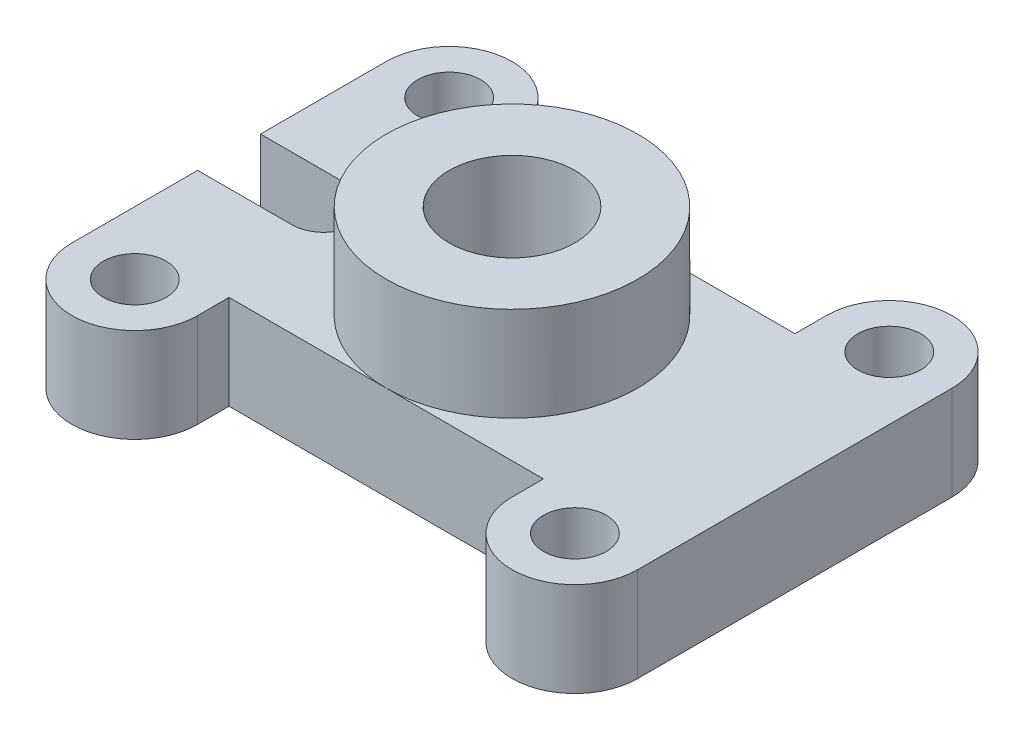
ISO-10303-21;
HEADER;
FILE_DESCRIPTION(('STEP AP214'),'2;1');
FILE_NAME('part.step','',(''),(''),'','','');
FILE_SCHEMA(('AUTOMOTIVE_DESIGN { 1 0 10303 214 1 1 1 1 }'));
ENDSEC;
DATA;
#1=APPLICATION_CONTEXT('core data for automotive mechanical design processes');
#2=APPLICATION_PROTOCOL_DEFINITION('international standard','automotive_design',2000,#1);
#3=PRODUCT_CONTEXT('',#1,'mechanical');
#4=PRODUCT('Part','Part','',(#3));
#5=PRODUCT_RELATED_PRODUCT_CATEGORY('part','',(#4));
#6=PRODUCT_DEFINITION_FORMATION('','',#4);
#7=PRODUCT_DEFINITION_CONTEXT('part definition',#1,'design');
#8=PRODUCT_DEFINITION('design','',#6,#7);
#9=PRODUCT_DEFINITION_SHAPE('','',#8);
#10=(LENGTH_UNIT() NAMED_UNIT(*) SI_UNIT(.MILLI.,.METRE.));
#11=(NAMED_UNIT(*) PLANE_ANGLE_UNIT() SI_UNIT($,.RADIAN.));
#12=(NAMED_UNIT(*) SI_UNIT($,.STERADIAN.) SOLID_ANGLE_UNIT());
#13=UNCERTAINTY_MEASURE_WITH_UNIT(LENGTH_MEASURE(1.E-05),#10,'distance_accuracy_value','');
#14=(GEOMETRIC_REPRESENTATION_CONTEXT(3) GLOBAL_UNCERTAINTY_ASSIGNED_CONTEXT((#13)) GLOBAL_UNIT_ASSIGNED_CONTEXT((#10,
#11,#12)) REPRESENTATION_CONTEXT('',''));
#15=CARTESIAN_POINT('',(0.,0.,0.));
#16=DIRECTION('',(0.,0.,1.));
#17=DIRECTION('',(1.,0.,0.));
#18=AXIS2_PLACEMENT_3D('',#15,#16,#17);
#19=CARTESIAN_POINT('',(0.,0.,0.));
#20=DIRECTION('',(0.,1.,0.));
#21=DIRECTION('',(0.,0.,1.));
#22=AXIS2_PLACEMENT_3D('',#19,#20,#21);
#23=PLANE('',#22);
#24=CARTESIAN_POINT('',(0.,0.,0.));
#25=DIRECTION('',(0.,1.,0.));
#26=DIRECTION('',(0.,0.,1.));
#27=AXIS2_PLACEMENT_3D('',#24,#25,#26);
#28=CIRCLE('',#27,20.);
#29=CARTESIAN_POINT('',(0.,0.,20.));
#30=VERTEX_POINT('',#29);
#31=CARTESIAN_POINT('',(0.,0.,-19.9999999999999));
#32=VERTEX_POINT('',#31);
#33=EDGE_CURVE('E55',#30,#32,#28,.T.);
#34=ORIENTED_EDGE('',*,*,#33,.F.);
#35=DIRECTION('',(1.,0.,0.));
#36=VECTOR('',#35,1.);
#37=CARTESIAN_POINT('',(0.,0.,19.9999999999999));
#38=LINE('',#37,#36);
#39=CARTESIAN_POINT('',(25.,0.,20.));
#40=VERTEX_POINT('',#39);
#41=EDGE_CURVE('E250',#30,#40,#38,.T.);
#42=ORIENTED_EDGE('',*,*,#41,.T.);
#43=DIRECTION('',(0.,0.,-1.));
#44=VECTOR('',#43,1.);
#45=CARTESIAN_POINT('',(25.,0.,0.));
#46=LINE('',#45,#44);
#47=CARTESIAN_POINT('',(25.,0.,25.));
#48=VERTEX_POINT('',#47);
#49=EDGE_CURVE('E183',#48,#40,#46,.T.);
#50=ORIENTED_EDGE('',*,*,#49,.F.);
#51=CARTESIAN_POINT('',(35.,0.,25.));
#52=DIRECTION('',(0.,1.,0.));
#53=DIRECTION('',(0.,0.,1.));
#54=AXIS2_PLACEMENT_3D('',#51,#52,#53);
#55=CIRCLE('',#54,10.);
#56=CARTESIAN_POINT('',(45.,0.,25.));
#57=VERTEX_POINT('',#56);
#58=EDGE_CURVE('E124',#57,#48,#55,.F.);
#59=ORIENTED_EDGE('',*,*,#58,.F.);
#60=DIRECTION('',(0.,0.,1.));
#61=VECTOR('',#60,1.);
#62=CARTESIAN_POINT('',(45.,0.,0.));
#63=LINE('',#62,#61);
#64=CARTESIAN_POINT('',(45.,0.,-25.));
#65=VERTEX_POINT('',#64);
#66=EDGE_CURVE('E213',#65,#57,#63,.T.);
#67=ORIENTED_EDGE('',*,*,#66,.F.);
#68=CARTESIAN_POINT('',(35.,0.,-25.));
#69=DIRECTION('',(0.,1.,0.));
#70=DIRECTION('',(0.,0.,1.));
#71=AXIS2_PLACEMENT_3D('',#68,#69,#70);
#72=CIRCLE('',#71,10.);
#73=CARTESIAN_POINT('',(25.,0.,-25.));
#74=VERTEX_POINT('',#73);
#75=EDGE_CURVE('E216',#65,#74,#72,.T.);
#76=ORIENTED_EDGE('',*,*,#75,.T.);
#77=DIRECTION('',(0.,0.,1.));
#78=VECTOR('',#77,1.);
#79=CARTESIAN_POINT('',(25.,0.,0.));
#80=LINE('',#79,#78);
#81=CARTESIAN_POINT('',(25.,0.,-20.));
#82=VERTEX_POINT('',#81);
#83=EDGE_CURVE('E218',#74,#82,#80,.T.);
#84=ORIENTED_EDGE('',*,*,#83,.T.);
#85=DIRECTION('',(1.,0.,0.));
#86=VECTOR('',#85,1.);
#87=CARTESIAN_POINT('',(0.,0.,-19.9999999999999));
#88=LINE('',#87,#86);
#89=EDGE_CURVE('E225',#32,#82,#88,.T.);
#90=ORIENTED_EDGE('',*,*,#89,.F.);
#91=EDGE_LOOP('',(#34,#42,#50,#59,#67,#76,#84,#90));
#92=FACE_BOUND('',#91,.T.);
#93=CARTESIAN_POINT('',(35.,0.,-25.));
#94=DIRECTION('',(0.,1.,0.));
#95=DIRECTION('',(0.,0.,1.));
#96=AXIS2_PLACEMENT_3D('',#93,#94,#95);
#97=CIRCLE('',#96,5.);
#98=CARTESIAN_POINT('',(35.,0.,-20.));
#99=VERTEX_POINT('',#98);
#100=EDGE_CURVE('E210',#99,#99,#97,.T.);
#101=ORIENTED_EDGE('',*,*,#100,.F.);
#102=EDGE_LOOP('',(#101));
#103=FACE_BOUND('',#102,.T.);
#104=CARTESIAN_POINT('',(35.,0.,25.));
#105=DIRECTION('',(0.,1.,0.));
#106=DIRECTION('',(0.,0.,1.));
#107=AXIS2_PLACEMENT_3D('',#104,#105,#106);
#108=CIRCLE('',#107,5.);
#109=CARTESIAN_POINT('',(35.,0.,30.));
#110=VERTEX_POINT('',#109);
#111=EDGE_CURVE('E199',#110,#110,#108,.F.);
#112=ORIENTED_EDGE('',*,*,#111,.T.);
#113=EDGE_LOOP('',(#112));
#114=FACE_BOUND('',#113,.T.);
#115=ADVANCED_FACE('F41',(#92,#103,#114),#23,.T.);
#116=CARTESIAN_POINT('',(45.,-15.,0.));
#117=DIRECTION('',(-1.,0.,0.));
#118=DIRECTION('',(0.,0.,1.));
#119=AXIS2_PLACEMENT_3D('',#116,#117,#118);
#120=PLANE('',#119);
#121=ORIENTED_EDGE('',*,*,#66,.T.);
#122=DIRECTION('',(0.,1.,0.));
#123=VECTOR('',#122,1.);
#124=CARTESIAN_POINT('',(45.,-15.,25.));
#125=LINE('',#124,#123);
#126=CARTESIAN_POINT('',(45.,-15.,25.));
#127=VERTEX_POINT('',#126);
#128=EDGE_CURVE('E49',#127,#57,#125,.T.);
#129=ORIENTED_EDGE('',*,*,#128,.F.);
#130=DIRECTION('',(0.,0.,1.));
#131=VECTOR('',#130,1.);
#132=CARTESIAN_POINT('',(45.,-15.,0.));
#133=LINE('',#132,#131);
#134=CARTESIAN_POINT('',(45.,-15.,-25.));
#135=VERTEX_POINT('',#134);
#136=EDGE_CURVE('E287',#135,#127,#133,.T.);
#137=ORIENTED_EDGE('',*,*,#136,.F.);
#138=DIRECTION('',(0.,1.,0.));
#139=VECTOR('',#138,1.);
#140=CARTESIAN_POINT('',(45.,-15.,-25.));
#141=LINE('',#140,#139);
#142=EDGE_CURVE('E44',#135,#65,#141,.T.);
#143=ORIENTED_EDGE('',*,*,#142,.T.);
#144=EDGE_LOOP('',(#121,#129,#137,#143));
#145=FACE_BOUND('',#144,.T.);
#146=ADVANCED_FACE('F282',(#145),#120,.F.);
#147=CARTESIAN_POINT('',(35.,-15.,25.));
#148=DIRECTION('',(0.,1.,0.));
#149=DIRECTION('',(0.,0.,1.));
#150=AXIS2_PLACEMENT_3D('',#147,#148,#149);
#151=CYLINDRICAL_SURFACE('',#150,10.);
#152=ORIENTED_EDGE('',*,*,#58,.T.);
#153=DIRECTION('',(0.,1.,0.));
#154=VECTOR('',#153,1.);
#155=CARTESIAN_POINT('',(25.,-15.,25.));
#156=LINE('',#155,#154);
#157=CARTESIAN_POINT('',(25.,-15.,25.));
#158=VERTEX_POINT('',#157);
#159=EDGE_CURVE('E190',#158,#48,#156,.T.);
#160=ORIENTED_EDGE('',*,*,#159,.F.);
#161=CARTESIAN_POINT('',(35.,-15.,25.));
#162=DIRECTION('',(0.,1.,0.));
#163=DIRECTION('',(0.,0.,1.));
#164=AXIS2_PLACEMENT_3D('',#161,#162,#163);
#165=CIRCLE('',#164,10.);
#166=EDGE_CURVE('E66',#127,#158,#165,.F.);
#167=ORIENTED_EDGE('',*,*,#166,.F.);
#168=ORIENTED_EDGE('',*,*,#128,.T.);
#169=EDGE_LOOP('',(#152,#160,#167,#168));
#170=FACE_BOUND('',#169,.T.);
#171=ADVANCED_FACE('F315',(#170),#151,.T.);
#172=CARTESIAN_POINT('',(25.,-15.,0.));
#173=DIRECTION('',(1.,0.,0.));
#174=DIRECTION('',(0.,0.,-1.));
#175=AXIS2_PLACEMENT_3D('',#172,#173,#174);
#176=PLANE('',#175);
#177=ORIENTED_EDGE('',*,*,#49,.T.);
#178=DIRECTION('',(0.,1.,0.));
#179=VECTOR('',#178,1.);
#180=CARTESIAN_POINT('',(25.,-15.,20.));
#181=LINE('',#180,#179);
#182=CARTESIAN_POINT('',(25.,-15.,20.));
#183=VERTEX_POINT('',#182);
#184=EDGE_CURVE('E181',#183,#40,#181,.T.);
#185=ORIENTED_EDGE('',*,*,#184,.F.);
#186=DIRECTION('',(0.,0.,-1.));
#187=VECTOR('',#186,1.);
#188=CARTESIAN_POINT('',(25.,-15.,0.));
#189=LINE('',#188,#187);
#190=EDGE_CURVE('E174',#158,#183,#189,.T.);
#191=ORIENTED_EDGE('',*,*,#190,.F.);
#192=ORIENTED_EDGE('',*,*,#159,.T.);
#193=EDGE_LOOP('',(#177,#185,#191,#192));
#194=FACE_BOUND('',#193,.T.);
#195=ADVANCED_FACE('F184',(#194),#176,.F.);
#196=CARTESIAN_POINT('',(0.,-15.,19.9999999999999));
#197=DIRECTION('',(0.,0.,1.));
#198=DIRECTION('',(1.,0.,0.));
#199=AXIS2_PLACEMENT_3D('',#196,#197,#198);
#200=PLANE('',#199);
#201=CARTESIAN_POINT('',(-25.0000000000002,0.,19.9999999999998));
#202=VERTEX_POINT('',#201);
#203=EDGE_CURVE('E253',#202,#30,#38,.T.);
#204=ORIENTED_EDGE('',*,*,#203,.F.);
#205=DIRECTION('',(0.,1.,0.));
#206=VECTOR('',#205,1.);
#207=CARTESIAN_POINT('',(-25.0000000000002,-15.,19.9999999999998));
#208=LINE('',#207,#206);
#209=CARTESIAN_POINT('',(-25.0000000000002,-15.,19.9999999999998));
#210=VERTEX_POINT('',#209);
#211=EDGE_CURVE('E188',#210,#202,#208,.T.);
#212=ORIENTED_EDGE('',*,*,#211,.F.);
#213=DIRECTION('',(1.,0.,0.));
#214=VECTOR('',#213,1.);
#215=CARTESIAN_POINT('',(0.,-15.,19.9999999999999));
#216=LINE('',#215,#214);
#217=EDGE_CURVE('E176',#210,#183,#216,.T.);
#218=ORIENTED_EDGE('',*,*,#217,.T.);
#219=ORIENTED_EDGE('',*,*,#184,.T.);
#220=ORIENTED_EDGE('',*,*,#41,.F.);
#221=EDGE_LOOP('',(#204,#212,#218,#219,#220));
#222=FACE_BOUND('',#221,.T.);
#223=ADVANCED_FACE('F192',(#222),#200,.T.);
#224=CARTESIAN_POINT('',(-25.0000000000007,-15.,7.28583859910253E-13));
#225=DIRECTION('',(1.,0.,0.));
#226=DIRECTION('',(0.,0.,-1.));
#227=AXIS2_PLACEMENT_3D('',#224,#225,#226);
#228=PLANE('',#227);
#229=DIRECTION('',(0.,0.,-1.));
#230=VECTOR('',#229,1.);
#231=CARTESIAN_POINT('',(-25.0000000000007,0.,7.28583859910253E-13));
#232=LINE('',#231,#230);
#233=CARTESIAN_POINT('',(-25.,0.,25.));
#234=VERTEX_POINT('',#233);
#235=EDGE_CURVE('E247',#234,#202,#232,.T.);
#236=ORIENTED_EDGE('',*,*,#235,.F.);
#237=DIRECTION('',(0.,1.,0.));
#238=VECTOR('',#237,1.);
#239=CARTESIAN_POINT('',(-25.,-15.,25.));
#240=LINE('',#239,#238);
#241=CARTESIAN_POINT('',(-25.,-15.,25.));
#242=VERTEX_POINT('',#241);
#243=EDGE_CURVE('E259',#242,#234,#240,.T.);
#244=ORIENTED_EDGE('',*,*,#243,.F.);
#245=DIRECTION('',(0.,0.,-1.));
#246=VECTOR('',#245,1.);
#247=CARTESIAN_POINT('',(-25.0000000000007,-15.,7.28583859910253E-13));
#248=LINE('',#247,#246);
#249=EDGE_CURVE('E194',#242,#210,#248,.T.);
#250=ORIENTED_EDGE('',*,*,#249,.T.);
#251=ORIENTED_EDGE('',*,*,#211,.T.);
#252=EDGE_LOOP('',(#236,#244,#250,#251));
#253=FACE_BOUND('',#252,.T.);
#254=ADVANCED_FACE('F582',(#253),#228,.T.);
#255=CARTESIAN_POINT('',(-35.,-15.,25.));
#256=DIRECTION('',(0.,1.,0.));
#257=DIRECTION('',(0.,0.,1.));
#258=AXIS2_PLACEMENT_3D('',#255,#256,#257);
#259=CYLINDRICAL_SURFACE('',#258,9.99999999999999);
#260=CARTESIAN_POINT('',(-35.,0.,25.));
#261=DIRECTION('',(0.,1.,0.));
#262=DIRECTION('',(0.,0.,1.));
#263=AXIS2_PLACEMENT_3D('',#260,#261,#262);
#264=CIRCLE('',#263,9.99999999999999);
#265=CARTESIAN_POINT('',(-45.,0.,25.));
#266=VERTEX_POINT('',#265);
#267=EDGE_CURVE('E243',#266,#234,#264,.T.);
#268=ORIENTED_EDGE('',*,*,#267,.F.);
#269=DIRECTION('',(0.,1.,0.));
#270=VECTOR('',#269,1.);
#271=CARTESIAN_POINT('',(-45.,-15.,25.));
#272=LINE('',#271,#270);
#273=CARTESIAN_POINT('',(-45.,-15.,25.));
#274=VERTEX_POINT('',#273);
#275=EDGE_CURVE('E261',#274,#266,#272,.T.);
#276=ORIENTED_EDGE('',*,*,#275,.F.);
#277=CARTESIAN_POINT('',(-35.,-15.,25.));
#278=DIRECTION('',(0.,1.,0.));
#279=DIRECTION('',(0.,0.,1.));
#280=AXIS2_PLACEMENT_3D('',#277,#278,#279);
#281=CIRCLE('',#280,9.99999999999999);
#282=EDGE_CURVE('E195',#274,#242,#281,.T.);
#283=ORIENTED_EDGE('',*,*,#282,.T.);
#284=ORIENTED_EDGE('',*,*,#243,.T.);
#285=EDGE_LOOP('',(#268,#276,#283,#284));
#286=FACE_BOUND('',#285,.T.);
#287=ADVANCED_FACE('F391',(#286),#259,.T.);
#288=CARTESIAN_POINT('',(-45.,-15.,0.));
#289=DIRECTION('',(-1.,0.,0.));
#290=DIRECTION('',(0.,0.,1.));
#291=AXIS2_PLACEMENT_3D('',#288,#289,#290);
#292=PLANE('',#291);
#293=DIRECTION('',(0.,0.,1.));
#294=VECTOR('',#293,1.);
#295=CARTESIAN_POINT('',(-45.,0.,0.));
#296=LINE('',#295,#294);
#297=CARTESIAN_POINT('',(-45.,0.,5.));
#298=VERTEX_POINT('',#297);
#299=EDGE_CURVE('E244',#298,#266,#296,.T.);
#300=ORIENTED_EDGE('',*,*,#299,.F.);
#301=DIRECTION('',(0.,1.,0.));
#302=VECTOR('',#301,1.);
#303=CARTESIAN_POINT('',(-45.,-15.,5.));
#304=LINE('',#303,#302);
#305=CARTESIAN_POINT('',(-45.,-15.,5.));
#306=VERTEX_POINT('',#305);
#307=EDGE_CURVE('E263',#306,#298,#304,.T.);
#308=ORIENTED_EDGE('',*,*,#307,.F.);
#309=DIRECTION('',(0.,0.,1.));
#310=VECTOR('',#309,1.);
#311=CARTESIAN_POINT('',(-45.,-15.,0.));
#312=LINE('',#311,#310);
#313=EDGE_CURVE('E387',#306,#274,#312,.T.);
#314=ORIENTED_EDGE('',*,*,#313,.T.);
#315=ORIENTED_EDGE('',*,*,#275,.T.);
#316=EDGE_LOOP('',(#300,#308,#314,#315));
#317=FACE_BOUND('',#316,.T.);
#318=ADVANCED_FACE('F397',(#317),#292,.T.);
#319=CARTESIAN_POINT('',(0.,-15.,5.));
#320=DIRECTION('',(0.,0.,1.));
#321=DIRECTION('',(1.,0.,0.));
#322=AXIS2_PLACEMENT_3D('',#319,#320,#321);
#323=PLANE('',#322);
#324=DIRECTION('',(1.,0.,0.));
#325=VECTOR('',#324,1.);
#326=CARTESIAN_POINT('',(0.,0.,5.));
#327=LINE('',#326,#325);
#328=CARTESIAN_POINT('',(-30.,0.,5.));
#329=VERTEX_POINT('',#328);
#330=EDGE_CURVE('E239',#298,#329,#327,.T.);
#331=ORIENTED_EDGE('',*,*,#330,.T.);
#332=DIRECTION('',(0.,1.,0.));
#333=VECTOR('',#332,1.);
#334=CARTESIAN_POINT('',(-30.,-15.,5.));
#335=LINE('',#334,#333);
#336=CARTESIAN_POINT('',(-30.,-15.,5.));
#337=VERTEX_POINT('',#336);
#338=EDGE_CURVE('E264',#337,#329,#335,.T.);
#339=ORIENTED_EDGE('',*,*,#338,.F.);
#340=DIRECTION('',(1.,0.,0.));
#341=VECTOR('',#340,1.);
#342=CARTESIAN_POINT('',(0.,-15.,5.));
#343=LINE('',#342,#341);
#344=EDGE_CURVE('E383',#306,#337,#343,.T.);
#345=ORIENTED_EDGE('',*,*,#344,.F.);
#346=ORIENTED_EDGE('',*,*,#307,.T.);
#347=EDGE_LOOP('',(#331,#339,#345,#346));
#348=FACE_BOUND('',#347,.T.);
#349=ADVANCED_FACE('F405',(#348),#323,.F.);
#350=CARTESIAN_POINT('',(-30.,-15.,0.));
#351=DIRECTION('',(0.,1.,0.));
#352=DIRECTION('',(0.,0.,1.));
#353=AXIS2_PLACEMENT_3D('',#350,#351,#352);
#354=CYLINDRICAL_SURFACE('',#353,5.);
#355=CARTESIAN_POINT('',(-30.,0.,0.));
#356=DIRECTION('',(0.,1.,0.));
#357=DIRECTION('',(0.,0.,1.));
#358=AXIS2_PLACEMENT_3D('',#355,#356,#357);
#359=CIRCLE('',#358,5.);
#360=CARTESIAN_POINT('',(-30.,0.,-5.));
#361=VERTEX_POINT('',#360);
#362=EDGE_CURVE('E237',#329,#361,#359,.T.);
#363=ORIENTED_EDGE('',*,*,#362,.T.);
#364=DIRECTION('',(0.,1.,0.));
#365=VECTOR('',#364,1.);
#366=CARTESIAN_POINT('',(-30.,-15.,-5.));
#367=LINE('',#366,#365);
#368=CARTESIAN_POINT('',(-30.,-15.,-5.));
#369=VERTEX_POINT('',#368);
#370=EDGE_CURVE('E268',#369,#361,#367,.T.);
#371=ORIENTED_EDGE('',*,*,#370,.F.);
#372=CARTESIAN_POINT('',(-30.,-15.,0.));
#373=DIRECTION('',(0.,1.,0.));
#374=DIRECTION('',(0.,0.,1.));
#375=AXIS2_PLACEMENT_3D('',#372,#373,#374);
#376=CIRCLE('',#375,5.);
#377=EDGE_CURVE('E385',#337,#369,#376,.T.);
#378=ORIENTED_EDGE('',*,*,#377,.F.);
#379=ORIENTED_EDGE('',*,*,#338,.T.);
#380=EDGE_LOOP('',(#363,#371,#378,#379));
#381=FACE_BOUND('',#380,.T.);
#382=ADVANCED_FACE('F410',(#381),#354,.F.);
#383=CARTESIAN_POINT('',(0.,-15.,-5.));
#384=DIRECTION('',(0.,0.,1.));
#385=DIRECTION('',(1.,0.,0.));
#386=AXIS2_PLACEMENT_3D('',#383,#384,#385);
#387=PLANE('',#386);
#388=DIRECTION('',(1.,0.,0.));
#389=VECTOR('',#388,1.);
#390=CARTESIAN_POINT('',(0.,0.,-5.));
#391=LINE('',#390,#389);
#392=CARTESIAN_POINT('',(-45.,0.,-5.));
#393=VERTEX_POINT('',#392);
#394=EDGE_CURVE('E234',#393,#361,#391,.T.);
#395=ORIENTED_EDGE('',*,*,#394,.F.);
#396=DIRECTION('',(0.,1.,0.));
#397=VECTOR('',#396,1.);
#398=CARTESIAN_POINT('',(-45.,-15.,-5.));
#399=LINE('',#398,#397);
#400=CARTESIAN_POINT('',(-45.,-15.,-5.));
#401=VERTEX_POINT('',#400);
#402=EDGE_CURVE('E269',#401,#393,#399,.T.);
#403=ORIENTED_EDGE('',*,*,#402,.F.);
#404=DIRECTION('',(1.,0.,0.));
#405=VECTOR('',#404,1.);
#406=CARTESIAN_POINT('',(0.,-15.,-5.));
#407=LINE('',#406,#405);
#408=EDGE_CURVE('E377',#401,#369,#407,.T.);
#409=ORIENTED_EDGE('',*,*,#408,.T.);
#410=ORIENTED_EDGE('',*,*,#370,.T.);
#411=EDGE_LOOP('',(#395,#403,#409,#410));
#412=FACE_BOUND('',#411,.T.);
#413=ADVANCED_FACE('F412',(#412),#387,.T.);
#414=CARTESIAN_POINT('',(-45.,-15.,0.));
#415=DIRECTION('',(-1.,0.,0.));
#416=DIRECTION('',(0.,0.,1.));
#417=AXIS2_PLACEMENT_3D('',#414,#415,#416);
#418=PLANE('',#417);
#419=DIRECTION('',(0.,0.,1.));
#420=VECTOR('',#419,1.);
#421=CARTESIAN_POINT('',(-45.,0.,0.));
#422=LINE('',#421,#420);
#423=CARTESIAN_POINT('',(-45.,0.,-25.));
#424=VERTEX_POINT('',#423);
#425=EDGE_CURVE('E227',#424,#393,#422,.T.);
#426=ORIENTED_EDGE('',*,*,#425,.F.);
#427=DIRECTION('',(0.,1.,0.));
#428=VECTOR('',#427,1.);
#429=CARTESIAN_POINT('',(-45.,-15.,-25.));
#430=LINE('',#429,#428);
#431=CARTESIAN_POINT('',(-45.,-15.,-25.));
#432=VERTEX_POINT('',#431);
#433=EDGE_CURVE('E275',#432,#424,#430,.T.);
#434=ORIENTED_EDGE('',*,*,#433,.F.);
#435=DIRECTION('',(0.,0.,1.));
#436=VECTOR('',#435,1.);
#437=CARTESIAN_POINT('',(-45.,-15.,0.));
#438=LINE('',#437,#436);
#439=EDGE_CURVE('E376',#432,#401,#438,.T.);
#440=ORIENTED_EDGE('',*,*,#439,.T.);
#441=ORIENTED_EDGE('',*,*,#402,.T.);
#442=EDGE_LOOP('',(#426,#434,#440,#441));
#443=FACE_BOUND('',#442,.T.);
#444=ADVANCED_FACE('F415',(#443),#418,.T.);
#445=CARTESIAN_POINT('',(-35.,-15.,-25.));
#446=DIRECTION('',(0.,1.,0.));
#447=DIRECTION('',(0.,0.,1.));
#448=AXIS2_PLACEMENT_3D('',#445,#446,#447);
#449=CYLINDRICAL_SURFACE('',#448,10.);
#450=CARTESIAN_POINT('',(-35.,0.,-25.));
#451=DIRECTION('',(0.,1.,0.));
#452=DIRECTION('',(0.,0.,1.));
#453=AXIS2_PLACEMENT_3D('',#450,#451,#452);
#454=CIRCLE('',#453,10.);
#455=CARTESIAN_POINT('',(-25.,0.,-25.0000000000003));
#456=VERTEX_POINT('',#455);
#457=EDGE_CURVE('E230',#424,#456,#454,.F.);
#458=ORIENTED_EDGE('',*,*,#457,.T.);
#459=DIRECTION('',(0.,1.,0.));
#460=VECTOR('',#459,1.);
#461=CARTESIAN_POINT('',(-25.,-15.,-25.0000000000003));
#462=LINE('',#461,#460);
#463=CARTESIAN_POINT('',(-25.,-15.,-25.0000000000003));
#464=VERTEX_POINT('',#463);
#465=EDGE_CURVE('E273',#464,#456,#462,.T.);
#466=ORIENTED_EDGE('',*,*,#465,.F.);
#467=CARTESIAN_POINT('',(-35.,-15.,-25.));
#468=DIRECTION('',(0.,1.,0.));
#469=DIRECTION('',(0.,0.,1.));
#470=AXIS2_PLACEMENT_3D('',#467,#468,#469);
#471=CIRCLE('',#470,10.);
#472=EDGE_CURVE('E372',#432,#464,#471,.F.);
#473=ORIENTED_EDGE('',*,*,#472,.F.);
#474=ORIENTED_EDGE('',*,*,#433,.T.);
#475=EDGE_LOOP('',(#458,#466,#473,#474));
#476=FACE_BOUND('',#475,.T.);
#477=ADVANCED_FACE('F423',(#476),#449,.T.);
#478=CARTESIAN_POINT('',(-25.0000000000008,-15.,-7.6327832942975E-13));
#479=DIRECTION('',(-1.,0.,0.));
#480=DIRECTION('',(0.,0.,1.));
#481=AXIS2_PLACEMENT_3D('',#478,#479,#480);
#482=PLANE('',#481);
#483=DIRECTION('',(0.,0.,1.));
#484=VECTOR('',#483,1.);
#485=CARTESIAN_POINT('',(-25.0000000000008,0.,-7.6327832942975E-13));
#486=LINE('',#485,#484);
#487=CARTESIAN_POINT('',(-25.0000000000002,0.,-19.9999999999998));
#488=VERTEX_POINT('',#487);
#489=EDGE_CURVE('E229',#456,#488,#486,.T.);
#490=ORIENTED_EDGE('',*,*,#489,.T.);
#491=DIRECTION('',(0.,1.,0.));
#492=VECTOR('',#491,1.);
#493=CARTESIAN_POINT('',(-25.0000000000002,-15.,-19.9999999999998));
#494=LINE('',#493,#492);
#495=CARTESIAN_POINT('',(-25.0000000000002,-15.,-19.9999999999998));
#496=VERTEX_POINT('',#495);
#497=EDGE_CURVE('E280',#496,#488,#494,.T.);
#498=ORIENTED_EDGE('',*,*,#497,.F.);
#499=DIRECTION('',(0.,0.,1.));
#500=VECTOR('',#499,1.);
#501=CARTESIAN_POINT('',(-25.0000000000008,-15.,-7.6327832942975E-13));
#502=LINE('',#501,#500);
#503=EDGE_CURVE('E375',#464,#496,#502,.T.);
#504=ORIENTED_EDGE('',*,*,#503,.F.);
#505=ORIENTED_EDGE('',*,*,#465,.T.);
#506=EDGE_LOOP('',(#490,#498,#504,#505));
#507=FACE_BOUND('',#506,.T.);
#508=ADVANCED_FACE('F422',(#507),#482,.F.);
#509=CARTESIAN_POINT('',(0.,-15.,-19.9999999999999));
#510=DIRECTION('',(0.,0.,1.));
#511=DIRECTION('',(1.,0.,0.));
#512=AXIS2_PLACEMENT_3D('',#509,#510,#511);
#513=PLANE('',#512);
#514=EDGE_CURVE('E224',#488,#32,#88,.T.);
#515=ORIENTED_EDGE('',*,*,#514,.T.);
#516=ORIENTED_EDGE('',*,*,#89,.T.);
#517=DIRECTION('',(0.,1.,0.));
#518=VECTOR('',#517,1.);
#519=CARTESIAN_POINT('',(25.,-15.,-20.));
#520=LINE('',#519,#518);
#521=CARTESIAN_POINT('',(25.,-15.,-20.));
#522=VERTEX_POINT('',#521);
#523=EDGE_CURVE('E278',#522,#82,#520,.T.);
#524=ORIENTED_EDGE('',*,*,#523,.F.);
#525=DIRECTION('',(1.,0.,0.));
#526=VECTOR('',#525,1.);
#527=CARTESIAN_POINT('',(0.,-15.,-19.9999999999999));
#528=LINE('',#527,#526);
#529=EDGE_CURVE('E367',#496,#522,#528,.T.);
#530=ORIENTED_EDGE('',*,*,#529,.F.);
#531=ORIENTED_EDGE('',*,*,#497,.T.);
#532=EDGE_LOOP('',(#515,#516,#524,#530,#531));
#533=FACE_BOUND('',#532,.T.);
#534=ADVANCED_FACE('F344',(#533),#513,.F.);
#535=CARTESIAN_POINT('',(25.,-15.,0.));
#536=DIRECTION('',(-1.,0.,0.));
#537=DIRECTION('',(0.,0.,1.));
#538=AXIS2_PLACEMENT_3D('',#535,#536,#537);
#539=PLANE('',#538);
#540=ORIENTED_EDGE('',*,*,#83,.F.);
#541=DIRECTION('',(0.,1.,0.));
#542=VECTOR('',#541,1.);
#543=CARTESIAN_POINT('',(25.,-15.,-25.));
#544=LINE('',#543,#542);
#545=CARTESIAN_POINT('',(25.,-15.,-25.));
#546=VERTEX_POINT('',#545);
#547=EDGE_CURVE('E281',#546,#74,#544,.T.);
#548=ORIENTED_EDGE('',*,*,#547,.F.);
#549=DIRECTION('',(0.,0.,1.));
#550=VECTOR('',#549,1.);
#551=CARTESIAN_POINT('',(25.,-15.,0.));
#552=LINE('',#551,#550);
#553=EDGE_CURVE('E370',#546,#522,#552,.T.);
#554=ORIENTED_EDGE('',*,*,#553,.T.);
#555=ORIENTED_EDGE('',*,*,#523,.T.);
#556=EDGE_LOOP('',(#540,#548,#554,#555));
#557=FACE_BOUND('',#556,.T.);
#558=ADVANCED_FACE('F331',(#557),#539,.T.);
#559=CARTESIAN_POINT('',(-35.,-15.,-25.));
#560=DIRECTION('',(0.,1.,0.));
#561=DIRECTION('',(0.,0.,1.));
#562=AXIS2_PLACEMENT_3D('',#559,#560,#561);
#563=CYLINDRICAL_SURFACE('',#562,5.);
#564=CARTESIAN_POINT('',(-35.,-15.,-25.));
#565=DIRECTION('',(0.,1.,0.));
#566=DIRECTION('',(0.,0.,1.));
#567=AXIS2_PLACEMENT_3D('',#564,#565,#566);
#568=CIRCLE('',#567,5.);
#569=CARTESIAN_POINT('',(-35.,-15.,-20.));
#570=VERTEX_POINT('',#569);
#571=EDGE_CURVE('E359',#570,#570,#568,.F.);
#572=ORIENTED_EDGE('',*,*,#571,.T.);
#573=EDGE_LOOP('',(#572));
#574=FACE_BOUND('',#573,.T.);
#575=CARTESIAN_POINT('',(-35.,0.,-25.));
#576=DIRECTION('',(0.,1.,0.));
#577=DIRECTION('',(0.,0.,1.));
#578=AXIS2_PLACEMENT_3D('',#575,#576,#577);
#579=CIRCLE('',#578,5.);
#580=CARTESIAN_POINT('',(-35.,0.,-20.));
#581=VERTEX_POINT('',#580);
#582=EDGE_CURVE('E209',#581,#581,#579,.F.);
#583=ORIENTED_EDGE('',*,*,#582,.F.);
#584=EDGE_LOOP('',(#583));
#585=FACE_BOUND('',#584,.T.);
#586=ADVANCED_FACE('F332',(#574,#585),#563,.F.);
#587=CARTESIAN_POINT('',(35.,-15.,-25.));
#588=DIRECTION('',(0.,1.,0.));
#589=DIRECTION('',(0.,0.,1.));
#590=AXIS2_PLACEMENT_3D('',#587,#588,#589);
#591=CYLINDRICAL_SURFACE('',#590,5.);
#592=CARTESIAN_POINT('',(35.,-15.,-25.));
#593=DIRECTION('',(0.,1.,0.));
#594=DIRECTION('',(0.,0.,1.));
#595=AXIS2_PLACEMENT_3D('',#592,#593,#594);
#596=CIRCLE('',#595,5.);
#597=CARTESIAN_POINT('',(35.,-15.,-20.));
#598=VERTEX_POINT('',#597);
#599=EDGE_CURVE('E352',#598,#598,#596,.T.);
#600=ORIENTED_EDGE('',*,*,#599,.F.);
#601=EDGE_LOOP('',(#600));
#602=FACE_BOUND('',#601,.T.);
#603=ORIENTED_EDGE('',*,*,#100,.T.);
#604=EDGE_LOOP('',(#603));
#605=FACE_BOUND('',#604,.T.);
#606=ADVANCED_FACE('F334',(#602,#605),#591,.F.);
#607=CARTESIAN_POINT('',(-35.,-15.,25.));
#608=DIRECTION('',(0.,1.,0.));
#609=DIRECTION('',(0.,0.,1.));
#610=AXIS2_PLACEMENT_3D('',#607,#608,#609);
#611=CYLINDRICAL_SURFACE('',#610,5.);
#612=CARTESIAN_POINT('',(-35.,-15.,25.));
#613=DIRECTION('',(0.,1.,0.));
#614=DIRECTION('',(0.,0.,1.));
#615=AXIS2_PLACEMENT_3D('',#612,#613,#614);
#616=CIRCLE('',#615,5.);
#617=CARTESIAN_POINT('',(-35.,-15.,30.));
#618=VERTEX_POINT('',#617);
#619=EDGE_CURVE('E355',#618,#618,#616,.T.);
#620=ORIENTED_EDGE('',*,*,#619,.F.);
#621=EDGE_LOOP('',(#620));
#622=FACE_BOUND('',#621,.T.);
#623=CARTESIAN_POINT('',(-35.,0.,25.));
#624=DIRECTION('',(0.,1.,0.));
#625=DIRECTION('',(0.,0.,1.));
#626=AXIS2_PLACEMENT_3D('',#623,#624,#625);
#627=CIRCLE('',#626,5.);
#628=CARTESIAN_POINT('',(-35.,0.,30.));
#629=VERTEX_POINT('',#628);
#630=EDGE_CURVE('E201',#629,#629,#627,.T.);
#631=ORIENTED_EDGE('',*,*,#630,.T.);
#632=EDGE_LOOP('',(#631));
#633=FACE_BOUND('',#632,.T.);
#634=ADVANCED_FACE('F301',(#622,#633),#611,.F.);
#635=CARTESIAN_POINT('',(35.,-15.,25.));
#636=DIRECTION('',(0.,1.,0.));
#637=DIRECTION('',(0.,0.,1.));
#638=AXIS2_PLACEMENT_3D('',#635,#636,#637);
#639=CYLINDRICAL_SURFACE('',#638,5.);
#640=CARTESIAN_POINT('',(35.,-15.,25.));
#641=DIRECTION('',(0.,1.,0.));
#642=DIRECTION('',(0.,0.,1.));
#643=AXIS2_PLACEMENT_3D('',#640,#641,#642);
#644=CIRCLE('',#643,5.);
#645=CARTESIAN_POINT('',(35.,-15.,30.));
#646=VERTEX_POINT('',#645);
#647=EDGE_CURVE('E254',#646,#646,#644,.F.);
#648=ORIENTED_EDGE('',*,*,#647,.T.);
#649=EDGE_LOOP('',(#648));
#650=FACE_BOUND('',#649,.T.);
#651=ORIENTED_EDGE('',*,*,#111,.F.);
#652=EDGE_LOOP('',(#651));
#653=FACE_BOUND('',#652,.T.);
#654=ADVANCED_FACE('F43',(#650,#653),#639,.F.);
#655=CARTESIAN_POINT('',(35.,-15.,-25.));
#656=DIRECTION('',(0.,1.,0.));
#657=DIRECTION('',(0.,0.,1.));
#658=AXIS2_PLACEMENT_3D('',#655,#656,#657);
#659=CYLINDRICAL_SURFACE('',#658,10.);
#660=ORIENTED_EDGE('',*,*,#75,.F.);
#661=ORIENTED_EDGE('',*,*,#142,.F.);
#662=CARTESIAN_POINT('',(35.,-15.,-25.));
#663=DIRECTION('',(0.,1.,0.));
#664=DIRECTION('',(0.,0.,1.));
#665=AXIS2_PLACEMENT_3D('',#662,#663,#664);
#666=CIRCLE('',#665,10.);
#667=EDGE_CURVE('E364',#135,#546,#666,.T.);
#668=ORIENTED_EDGE('',*,*,#667,.T.);
#669=ORIENTED_EDGE('',*,*,#547,.T.);
#670=EDGE_LOOP('',(#660,#661,#668,#669));
#671=FACE_BOUND('',#670,.T.);
#672=ADVANCED_FACE('F292',(#671),#659,.T.);
#673=CARTESIAN_POINT('',(0.,-15.,0.));
#674=DIRECTION('',(0.,1.,0.));
#675=DIRECTION('',(0.,0.,1.));
#676=AXIS2_PLACEMENT_3D('',#673,#674,#675);
#677=PLANE('',#676);
#678=ORIENTED_EDGE('',*,*,#647,.F.);
#679=EDGE_LOOP('',(#678));
#680=FACE_BOUND('',#679,.T.);
#681=ORIENTED_EDGE('',*,*,#619,.T.);
#682=EDGE_LOOP('',(#681));
#683=FACE_BOUND('',#682,.T.);
#684=ORIENTED_EDGE('',*,*,#599,.T.);
#685=EDGE_LOOP('',(#684));
#686=FACE_BOUND('',#685,.T.);
#687=ORIENTED_EDGE('',*,*,#571,.F.);
#688=EDGE_LOOP('',(#687));
#689=FACE_BOUND('',#688,.T.);
#690=ORIENTED_EDGE('',*,*,#136,.T.);
#691=ORIENTED_EDGE('',*,*,#166,.T.);
#692=ORIENTED_EDGE('',*,*,#190,.T.);
#693=ORIENTED_EDGE('',*,*,#217,.F.);
#694=ORIENTED_EDGE('',*,*,#249,.F.);
#695=ORIENTED_EDGE('',*,*,#282,.F.);
#696=ORIENTED_EDGE('',*,*,#313,.F.);
#697=ORIENTED_EDGE('',*,*,#344,.T.);
#698=ORIENTED_EDGE('',*,*,#377,.T.);
#699=ORIENTED_EDGE('',*,*,#408,.F.);
#700=ORIENTED_EDGE('',*,*,#439,.F.);
#701=ORIENTED_EDGE('',*,*,#472,.T.);
#702=ORIENTED_EDGE('',*,*,#503,.T.);
#703=ORIENTED_EDGE('',*,*,#529,.T.);
#704=ORIENTED_EDGE('',*,*,#553,.F.);
#705=ORIENTED_EDGE('',*,*,#667,.F.);
#706=EDGE_LOOP('',(#690,#691,#692,#693,#694,#695,#696,#697,#698,#699,#700,#701,#702,#703,#704,#705));
#707=FACE_BOUND('',#706,.T.);
#708=ADVANCED_FACE('F175',(#680,#683,#686,#689,#707),#677,.F.);
#709=EDGE_CURVE('E11',#32,#30,#28,.T.);
#710=ORIENTED_EDGE('',*,*,#709,.F.);
#711=ORIENTED_EDGE('',*,*,#514,.F.);
#712=ORIENTED_EDGE('',*,*,#489,.F.);
#713=ORIENTED_EDGE('',*,*,#457,.F.);
#714=ORIENTED_EDGE('',*,*,#425,.T.);
#715=ORIENTED_EDGE('',*,*,#394,.T.);
#716=ORIENTED_EDGE('',*,*,#362,.F.);
#717=ORIENTED_EDGE('',*,*,#330,.F.);
#718=ORIENTED_EDGE('',*,*,#299,.T.);
#719=ORIENTED_EDGE('',*,*,#267,.T.);
#720=ORIENTED_EDGE('',*,*,#235,.T.);
#721=ORIENTED_EDGE('',*,*,#203,.T.);
#722=EDGE_LOOP('',(#710,#711,#712,#713,#714,#715,#716,#717,#718,#719,#720,#721));
#723=FACE_BOUND('',#722,.T.);
#724=ORIENTED_EDGE('',*,*,#630,.F.);
#725=EDGE_LOOP('',(#724));
#726=FACE_BOUND('',#725,.T.);
#727=ORIENTED_EDGE('',*,*,#582,.T.);
#728=EDGE_LOOP('',(#727));
#729=FACE_BOUND('',#728,.T.);
#730=ADVANCED_FACE('F300',(#723,#726,#729),#23,.T.);
#731=CARTESIAN_POINT('',(0.,15.,0.));
#732=DIRECTION('',(0.,1.,0.));
#733=DIRECTION('',(0.,0.,1.));
#734=AXIS2_PLACEMENT_3D('',#731,#732,#733);
#735=PLANE('',#734);
#736=CARTESIAN_POINT('',(0.,15.,0.));
#737=DIRECTION('',(0.,1.,0.));
#738=DIRECTION('',(0.,0.,1.));
#739=AXIS2_PLACEMENT_3D('',#736,#737,#738);
#740=CIRCLE('',#739,20.);
#741=CARTESIAN_POINT('',(0.,15.,20.));
#742=VERTEX_POINT('',#741);
#743=EDGE_CURVE('E204',#742,#742,#740,.T.);
#744=ORIENTED_EDGE('',*,*,#743,.T.);
#745=EDGE_LOOP('',(#744));
#746=FACE_BOUND('',#745,.T.);
#747=CARTESIAN_POINT('',(0.,15.,0.));
#748=DIRECTION('',(0.,1.,0.));
#749=DIRECTION('',(0.,0.,1.));
#750=AXIS2_PLACEMENT_3D('',#747,#748,#749);
#751=CIRCLE('',#750,10.);
#752=CARTESIAN_POINT('',(0.,15.,10.));
#753=VERTEX_POINT('',#752);
#754=EDGE_CURVE('E435',#753,#753,#751,.T.);
#755=ORIENTED_EDGE('',*,*,#754,.F.);
#756=EDGE_LOOP('',(#755));
#757=FACE_BOUND('',#756,.T.);
#758=ADVANCED_FACE('F318',(#746,#757),#735,.T.);
#759=CARTESIAN_POINT('',(0.,15.,0.));
#760=DIRECTION('',(0.,-1.,0.));
#761=DIRECTION('',(0.,0.,-1.));
#762=AXIS2_PLACEMENT_3D('',#759,#760,#761);
#763=CYLINDRICAL_SURFACE('',#762,20.);
#764=ORIENTED_EDGE('',*,*,#743,.F.);
#765=EDGE_LOOP('',(#764));
#766=FACE_BOUND('',#765,.T.);
#767=ORIENTED_EDGE('',*,*,#33,.T.);
#768=ORIENTED_EDGE('',*,*,#709,.T.);
#769=EDGE_LOOP('',(#767,#768));
#770=FACE_BOUND('',#769,.T.);
#771=ADVANCED_FACE('F323',(#766,#770),#763,.T.);
#772=CARTESIAN_POINT('',(0.,15.,0.));
#773=DIRECTION('',(0.,-1.,0.));
#774=DIRECTION('',(0.,0.,-1.));
#775=AXIS2_PLACEMENT_3D('',#772,#773,#774);
#776=CYLINDRICAL_SURFACE('',#775,10.);
#777=ORIENTED_EDGE('',*,*,#754,.T.);
#778=EDGE_LOOP('',(#777));
#779=FACE_BOUND('',#778,.T.);
#780=CARTESIAN_POINT('',(0.,0.,0.));
#781=DIRECTION('',(0.,1.,0.));
#782=DIRECTION('',(0.,0.,1.));
#783=AXIS2_PLACEMENT_3D('',#780,#781,#782);
#784=CIRCLE('',#783,10.);
#785=CARTESIAN_POINT('',(0.,0.,10.));
#786=VERTEX_POINT('',#785);
#787=EDGE_CURVE('E436',#786,#786,#784,.T.);
#788=ORIENTED_EDGE('',*,*,#787,.F.);
#789=EDGE_LOOP('',(#788));
#790=FACE_BOUND('',#789,.T.);
#791=ADVANCED_FACE('F312',(#779,#790),#776,.F.);
#792=ORIENTED_EDGE('',*,*,#787,.T.);
#793=EDGE_LOOP('',(#792));
#794=FACE_BOUND('',#793,.T.);
#795=ADVANCED_FACE('F307',(#794),#23,.T.);
#796=CLOSED_SHELL('',(#115,#146,#171,#195,#223,#254,#287,#318,#349,#382,#413,#444,#477,#508,
#534,#558,#586,#606,#634,#654,#672,#708,#730,#758,#771,#791,#795));
#797=MANIFOLD_SOLID_BREP('B2',#796);
#798=ADVANCED_BREP_SHAPE_REPRESENTATION('',(#18,#797),#14);
#799=SHAPE_DEFINITION_REPRESENTATION(#9,#798);
ENDSEC;
END-ISO-10303-21;
